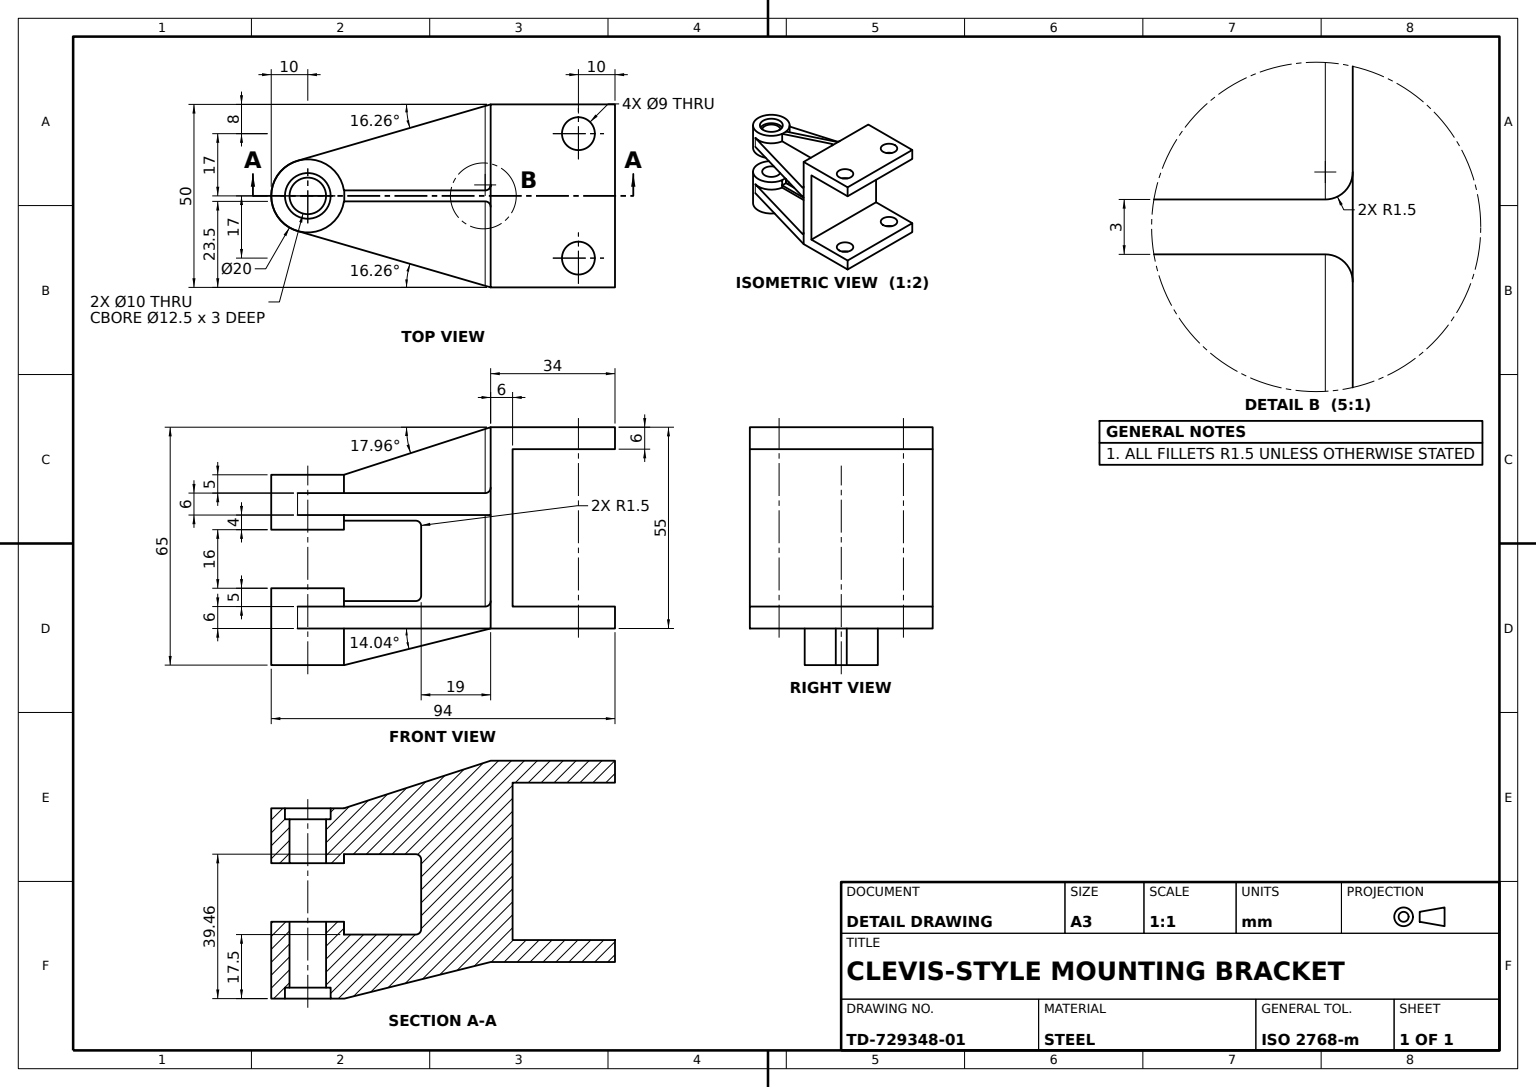
SolidWorks part; units mm, degrees
material "Plain Carbon Steel"
ref_plane "Front Plane" through (0, 0, 0) normal (0, 0, 1) x (1, 0, 0)
ref_plane "Top Plane" through (0, 0, 0) normal (0, 1, 0) x (1, 0, 0)
ref_plane "Right Plane" through (0, 0, 0) normal (1, 0, 0) x (0, 0, -1)
sketch "U-Channel Profile Sketch" plane through (0, 0, 0) normal (0, 0, 1) x (1, 0, 0)
  line L0 (0, 37.5) -> (0, 19.5)
  line L1 (0, 37.5) -> (34, 37.5)
  line L2 (34, 37.5) -> (34, 31.5)
  line L3 (34, 31.5) -> (6, 31.5)
  line L4 (6, 31.5) -> (6, -11.5)
  line L5 (6, -11.5) -> (34, -11.5)
  line L6 (34, -11.5) -> (34, -17.5)
  line L7 (34, -17.5) -> (0, -17.5)
  line L8 (0, 19.5) -> (-50, 19.5)
  line L9 (-50, 19.5) -> (-50, 13.5)
  line L10 (-50, 13.5) -> (0, 13.5)
  line L11 (0, -17.5) -> (-50, -17.5)
  line L12 (-50, -17.5) -> (-50, -11.5)
  line L13 (-50, -11.5) -> (0, -11.5)
  line L14 (0, 13.5) -> (0, -11.5)
  dimension "D1" = 55
  dimension "D2" = 6
  dimension "D3" = 6
  dimension "D4" = 6
  dimension "D5" = 34
  dimension "D6" = 34
  dimension "D7" = 50
  dimension "D8" = 50
  dimension "D9" = 37
  dimension "D10" = 6
  dimension "D11" = 37.5
extrude "U-Channel Base" add sketch "U-Channel Profile Sketch" along normal mid plane 50
sketch "Upper Lug Boss Sketch Ø20" plane through (0, 19.5, 0) normal (0, 1, 0) x (1, 0, 0)
  line L0 (-50, -25) -> (-50, 25) construction
  circle A0 centre (-50, 0) radius 10
  dimension "D1" = 20
extrude "Upper Lug Boss Ø20" add sketch "Upper Lug Boss Sketch Ø20" against normal blind 10
sketch "Upper Lug Pad Sketch" plane through (0, 19.5, 0) normal (0, 1, 0) x (1, 0, 0)
  circle A0 centre (-50, 0) radius 10
  dimension "D1" = 20
extrude "Upper Lug Pad" add sketch "Upper Lug Pad Sketch" along normal blind 5
sketch "Upper Counterbore Sketch Ø12.5" plane through (0, 24.5, 0) normal (0, 1, 0) x (1, 0, 0)
  circle A0 centre (-50, 0) radius 6.25
  dimension "D1" = 12.5
extrude "Upper Counterbore Ø12.5" cut sketch "Upper Counterbore Sketch Ø12.5" against normal blind 3
sketch "Upper Lug Hole Sketch Ø10" plane through (0, 21.5, 0) normal (0, 1, 0) x (1, 0, 0)
  circle A0 centre (-50, 0) radius 5
  dimension "D1" = 10
extrude "Upper Lug Hole Ø10" cut sketch "Upper Lug Hole Sketch Ø10" against normal blind 12
sketch "Lower Lug Pad Sketch" plane through (0, -17.5, 0) normal (0, -1, 0) x (1, 0, 0)
  line L0 (-50, 25) -> (-50, -25) construction
  circle A0 centre (-50, 0) radius 10
  dimension "D1" = 20
extrude "Lower Lug Pad" add sketch "Lower Lug Pad Sketch" against normal blind 11
sketch "Lower Lug Boss Sketch Ø20" plane through (0, -17.5, 0) normal (0, -1, 0) x (1, 0, 0)
  circle A0 centre (-50, 0) radius 10
  dimension "D1" = 20
extrude "Lower Lug Boss Ø20" add sketch "Lower Lug Boss Sketch Ø20" along normal blind 10
sketch "Lower Counterbore Sketch Ø12.5" plane through (0, -27.5, 0) normal (0, -1, 0) x (1, 0, 0)
  circle A0 centre (-50, 0) radius 6.25
  dimension "D1" = 12.5
extrude "Lower Counterbore Ø12.5" cut sketch "Lower Counterbore Sketch Ø12.5" against normal blind 3
sketch "Lower Lug Hole Sketch Ø10" plane through (0, -24.5, 0) normal (0, -1, 0) x (1, 0, 0)
  circle A0 centre (-50, 0) radius 5
  dimension "D1" = 10
extrude "Lower Lug Hole Ø10" cut sketch "Lower Lug Hole Sketch Ø10" against normal blind 18
sketch "Upper Gusset Sketch" plane through (0, 19.5, 0) normal (0, 1, 0) x (1, 0, 0)
  line L0 (0, 25) -> (-50, 10.4167)
  line L1 (-52.8, -9.6) -> (-52.8, -25)
  line L2 (-50, -10.4167) -> (0, -25)
  line L3 (-52.8, -25) -> (0, -25)
  line L4 (0, 25) -> (-52.8, 25)
  line L5 (-52.8, 25) -> (-52.8, 9.6)
  line L6 (-50, 10.4167) -> (-50, 10)
  line L7 (-50, 10) -> (-50, 25) construction
  line L8 (-50, 10) -> (-52.8, 9.6)
  line L9 (-52.8, -9.6) -> (-50, -10)
  line L10 (-50, -10) -> (-50, -10.4167)
  line L11 (-50, -25) -> (-50, -10) construction
  circle A0 centre (-50, 0) radius 10 construction
extrude "Upper Gusset" add sketch "Upper Gusset Sketch" against normal blind 6
sketch "Upper Gusset Trim Sketch" plane through (0, 19.5, 0) normal (0, 1, 0) x (1, 0, 0)
  line L0 (0, 25) -> (-52.8, 9.6)
  line L1 (-52.8, 9.6) -> (-52.8, 25)
  line L2 (-52.8, 25) -> (0, 25)
  line L3 (0, -25) -> (-52.8, -9.6)
  line L4 (-52.8, -9.6) -> (-52.8, -25)
  line L5 (-52.8, -25) -> (0, -25)
  circle A0 centre (-50, 0) radius 10 construction
extrude "Upper Gusset Trim" cut sketch "Upper Gusset Trim Sketch" against normal blind 6
sketch "Lower Gusset Sketch" plane through (0, -17.5, 0) normal (0, -1, 0) x (1, 0, 0)
  line L1 (0, 25) -> (-50, 10.4167)
  line L2 (-50, -25) -> (34, -25) construction
  line L5 (-52.8, 9.6) -> (-52.8, 25)
  line L6 (-52.8, 25) -> (0, 25)
  line L7 (0, -25) -> (-50, -10.4167)
  line L9 (-52.8, -9.6) -> (-52.8, -25)
  line L10 (-52.8, -25) -> (0, -25)
  line L11 (-50, -10) -> (-50, -10.4167)
  line L12 (-52.8, -9.6) -> (-50, -10)
  line L13 (-52.8, 9.6) -> (-50, 10)
  line L14 (-50, 10) -> (-50, 10.4167)
  line L15 (-50, 25) -> (-50, 10) construction
  circle A0 centre (-50, 0) radius 10 construction
  arc A1 (-50, -10) -> (-50, 10) centre (-50, 0) ccw construction
extrude "Lower Gusset" add sketch "Lower Gusset Sketch" against normal blind 6
sketch "Lower Gusset Trim Sketch" plane through (0, -17.5, 0) normal (0, -1, 0) x (1, 0, 0)
  line L2 (0, 25) -> (-52.8, 9.6)
  line L3 (-52.8, 9.6) -> (-52.8, 25)
  line L4 (-52.8, 25) -> (0, 25)
  line L5 (0, -25) -> (-52.8, -9.6)
  line L6 (-52.8, -9.6) -> (-52.8, -25)
  line L7 (-52.8, -25) -> (0, -25)
extrude "Lower Gusset Trim" cut sketch "Lower Gusset Trim Sketch" against normal blind 6
sketch "Back Plate Sketch" plane through (0, 0, 0) normal (0, 0, 1) x (1, 0, 0)
  line L0 (0, 0) -> (0, 32.5)
  line L1 (0, 0) -> (0, -32.5)
  line L2 (0, 32.5) -> (-40.1236, 32.5)
  line L3 (-40.1236, 32.5) -> (-40.1236, -32.5)
  line L4 (-40.1236, -32.5) -> (0, -32.5)
  dimension "D1" = 32.5
  dimension "D2" = 32.5
  dimension "D3" = 65
  dimension "D4" = 40.1236
extrude "Back Plate" add sketch "Back Plate Sketch" along normal mid plane 3 separate body
sketch "Back Plate Lower Relief Sketch" plane through (0, 0, 1.5) normal (0, 0, 1) x (1, 0, 0)
  line L0 (-40, -27.5) -> (0, -17.5)
  line L1 (0, -32.5) -> (0, 32.5) construction
  line L2 (-52.8, -17.5) -> (0, -17.5) construction
  line L3 (0, -17.5) -> (0, -32.5)
  line L4 (-40.1236, -32.5) -> (0, -32.5) construction
  line L5 (-40, -27.5) -> (-40.1236, -32.5)
  line L6 (-40.1236, -32.5) -> (0, -32.5)
extrude "Back Plate Lower Relief" cut sketch "Back Plate Lower Relief Sketch" against normal blind 3
sketch "Lower Lug Relief Sketch" plane through (-40.1236, 0, 0) normal (-1, 0, 0) x (0, 0, 1)
  line L3 (-1.5, -32.5) -> (1.5, -32.5)
  line L4 (1.5, 32.5) -> (1.5, -32.5) construction
  line L5 (1.5, -32.5) -> (-1.5, -32.5) construction
  line L6 (1.5, -32.5) -> (1.5, -27.5)
  line L7 (-10, -27.5) -> (10, -27.5) construction
  line L8 (1.5, -27.5) -> (-1.5, -27.5)
  line L9 (-1.5, -27.5) -> (-1.5, -32.5)
extrude "Lower Lug Relief" cut sketch "Lower Lug Relief Sketch" against normal blind 3
sketch "Back Plate Upper Relief Sketch" plane through (0, 0, 1.5) normal (0, 0, 1) x (1, 0, 0)
  line L0 (0, 32.5) -> (0, 19.5)
  line L1 (0, 37.5) -> (0, 19.5) construction
  line L2 (0, -17.5) -> (0, 32.5) construction
  line L3 (0, 19.5) -> (-40.1236, 19.5)
  line L4 (0, 19.5) -> (-52.8, 19.5) construction
  line L5 (-40.1236, 32.5) -> (-40.1236, -27.5) construction
  line L6 (-40.1236, 19.5) -> (-40.1236, 32.5)
  line L7 (0, 32.5) -> (-40.1236, 32.5) construction
  line L8 (-40.1236, 32.5) -> (0, 32.5)
extrude "Back Plate Upper Relief" cut sketch "Back Plate Upper Relief Sketch" against normal blind 3
sketch "Back Plate Edge Trim Sketch" plane through (0, 0, 1.5) normal (0, 0, 1) x (1, 0, 0)
  line L1 (-40.1236, 19.5) -> (-40.1236, -27.5) construction
  line L2 (-40.1236, 11.9641) -> (-19, 11.9641)
  line L3 (-19, 11.9641) -> (-19, -10)
  line L4 (-19, -10) -> (-40.1236, -10)
  line L6 (-40, -27.5) -> (-40.1236, -27.5) construction
  line L12 (-40.1236, 11.9641) -> (-40.1236, -10)
  dimension "D1" = 21.1236
  dimension "D2" = 17.5
  dimension "D3" = 39.4641
extrude "Back Plate Edge Trim" cut sketch "Back Plate Edge Trim Sketch" against normal blind 3
sketch "Web Sketch" plane through (0, 19.5, 0) normal (0, 1, 0) x (1, 0, 0)
  line L0 (-40.1236, -1.5) -> (0, -1.5)
  line L3 (0, -1.5) -> (0, 1.5)
  line L4 (-40.1236, -1.5) -> (-40.1236, 1.5)
  line L6 (-40.1236, 1.5) -> (0, 1.5)
extrude "Web" add sketch "Web Sketch" along normal blind 18
sketch "Web Chamfer Cut Sketch" plane through (0, 0, 1.5) normal (0, 0, 1) x (1, 0, 0)
  line L0 (0, 37.5) -> (-40.1131, 24.5)
  line L1 (-40.1131, 24.5) -> (-40.1236, 37.5)
  line L2 (-40.1236, 37.5) -> (0, 37.5)
extrude "Web Chamfer Cut" cut sketch "Web Chamfer Cut Sketch" against normal blind 3
sketch "Web Face Trim Sketch" plane through (-40.1236, 0, 0) normal (-1, 0, 0) x (0, 0, 1)
  line L0 (-1.5, 37.5) -> (1.5, 37.5)
  line L1 (1.5, 37.5) -> (1.5, 24.5)
  line L2 (10, 24.5) -> (-10, 24.5) construction
  line L3 (-1.5, 24.5) -> (1.5, 24.5) construction
  line L4 (1.5, 24.5) -> (-1.5, 24.5)
  line L5 (-1.5, 24.5) -> (-1.5, 37.5)
extrude "Web Face Trim 0.1" cut sketch "Web Face Trim Sketch" against normal blind 0.1
sketch "Flange Mounting Holes Sketch" plane through (0, 37.5, 0) normal (0, 1, 0) x (1, 0, 0)
  line L0 (34, -25) -> (34, 25) construction
  line L1 (34, -25) -> (0, -25) construction
  line L2 (34, 25) -> (0, 25) construction
  circle A0 centre (24, 17) radius 4.5
  circle A1 centre (24, -17) radius 4.5
  dimension "D3" = 9
  dimension "D4" = 9
  dimension "D1" = 10
  dimension "D2" = 10
  dimension "D5" = 8
  dimension "D6" = 8
  dimension "D7" = 34
extrude "Flange Mounting Holes 4x" cut sketch "Flange Mounting Holes Sketch" against normal blind 59.1
fillet "Edge Fillet R1.5" radius 1.5 10 edges at (-19, 11.9641, 0) (0, 1, -1.5) (0, -11.5, -13.25) (0, 19.5, -13.25) (0, 28.5, -1.5) (-19, -10, 0) (0, 1, 1.5) (0, 28.5, 1.5) (0, 19.5, 13.25) (0, -11.5, 13.25)
